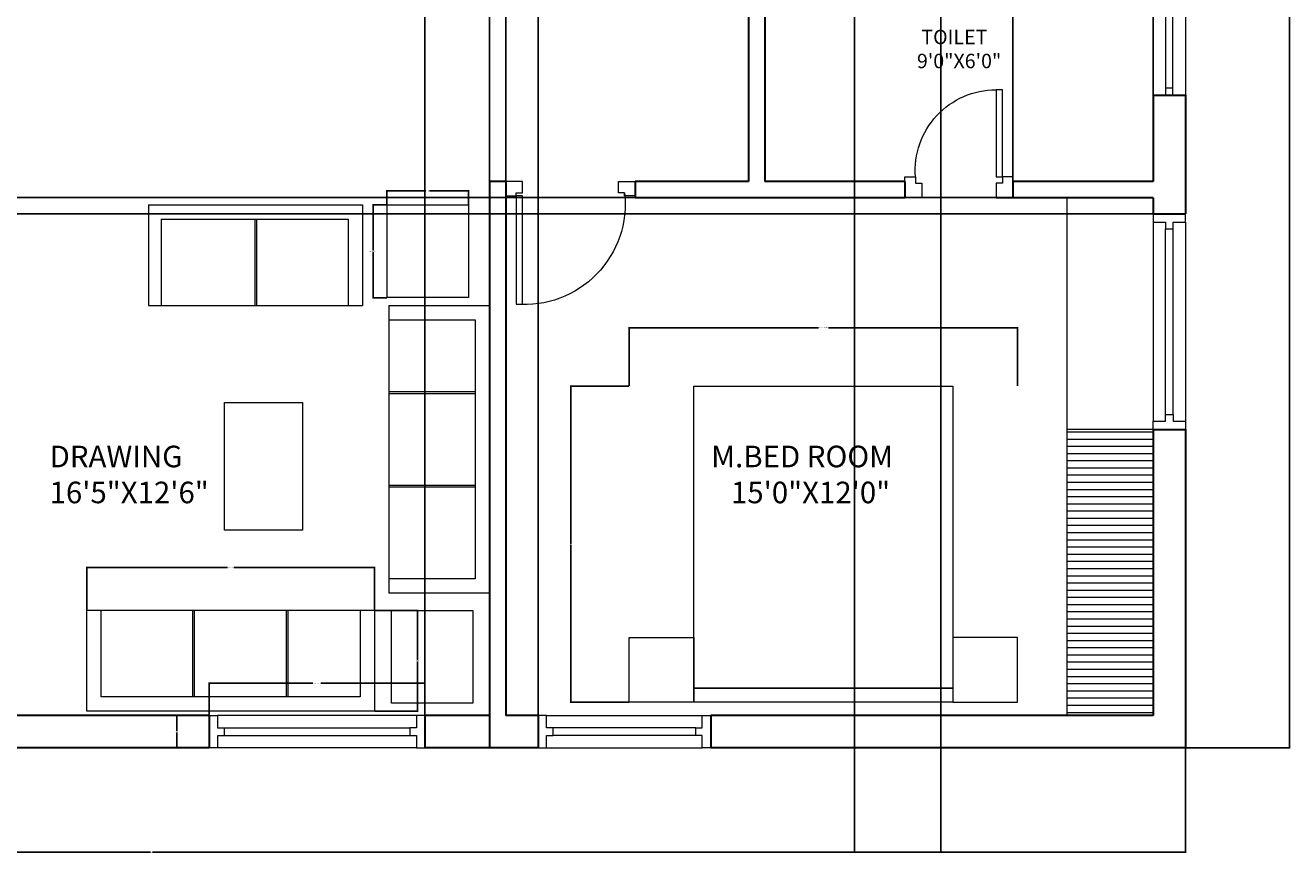
# Model space of a CAD drawing. Units: inches. Extents: x 2134 to 2768, y 715 to 1206.
# Tile 3 of 4: x 2416 to 2768, y 715 to 945. Entities that reach past the tile are written whole.
import ezdxf

# ---------------------------------------------------------------- set-up
doc = ezdxf.new("R2010")
doc.units = ezdxf.units.IN
for name, color, linetype, lineweight in [('A-ANNO-DIMS', 2, 'Continuous', 18), ('A-AREA-IDEN', 7, 'Continuous', 18), ('A-DOOR', 251, 'Continuous', 13), ('A-FLOR-CASE', 251, 'Continuous', 13), ('A-FLOR-CASE-PATT', 252, 'Continuous', 9), ('A-FURN', 251, 'Continuous', 13), ('A-WALL', 7, 'Continuous', 30), ('A-WINDOW', 251, 'Continuous', 13)]:
    doc.layers.add(name, color=color, linetype=linetype, lineweight=lineweight)
doc.styles.get("Standard").update_dxf_attribs({"font": 'arial.ttf'})
doc.dimstyles.get("Standard").update_dxf_attribs({"dimtxt": 0.18, "dimasz": 0.18, "dimexe": 0.18, "dimexo": 0.0625, "dimgap": 0.09, "dimtad": 0, "dimtih": 1, "dimtoh": 1, "dimdec": 4, "dimzin": 0, "dimdsep": 46, "dimtxsty": 'Standard', "dimcen": 0.09, "dimadec": 0, "dimazin": 0, "dimtfac": 1, "dimtdec": 4, "dimtofl": 0, "dimtmove": 0, "dimatfit": 3, "dimfxl": 1, "dimtolj": 1, "dimtzin": 0, "dimarcsym": 0})

# ---------------------------------------------------------------- blocks, each defined once
blk = doc.blocks.new('2 feet 6 inch door')
at = {"layer": 'A-DOOR'}
for points in [[(2.92, 5.83), (2.92, 30), (4.67, 30), (4.67, 5.83)], [(2.92, 4.08), (4.67, 4.08), (4.67, 0), (0, 0), (0, 5.83), (2.92, 5.83)], [(27.08, 5.83), (27.08, 4.08), (25.33, 4.08), (25.33, 0), (30, 0), (30, 5.83)]]:
    blk.add_lwpolyline(points, close=True, dxfattribs=at)
at = {"layer": 'A-DOOR', "ltscale": 0.1}
blk.add_arc((4.67, 7.52), 22.48, 355.6972, 90, dxfattribs=at)
blk = doc.blocks.new('ARCHITRAVE')
at = {"layer": 'A-DOOR'}
for p, q in [((0, 0), (0, 4)), ((0, 3.99), (2.92, 3.99)), ((2.92, 3.99), (2.92, 3.17)), ((4.67, 0), (0, 0)), ((2.92, 3.17), (4.67, 3.17)), ((4.67, 3.17), (4.67, 0))]:
    blk.add_line(p, q, dxfattribs=at)
blk = doc.blocks.new('3 FEET DOOR')
at = {"layer": 'A-DOOR'}
blk.add_lwpolyline([(-34.02, 3.98), (-34.02, 34.15), (-32.27, 34.15), (-32.27, 3.98)], close=True, dxfattribs=at)
at = {"layer": 'A-DOOR', "ltscale": 0.1}
blk.add_arc((-31.74, 6.19), 28.05, 353.8214, 94.662, dxfattribs=at)
at = {"layer": 'A-DOOR'}
blk.add_blockref('ARCHITRAVE', (-36.91, 0), dxfattribs=at)
at = {"layer": 'A-DOOR', "xscale": -1}
blk.add_blockref('ARCHITRAVE', (-0.93, 0), dxfattribs=at)
blk = doc.blocks.new('bed')
at = {"layer": 'A-FURN'}
for points in [[(3369.68, 925.24), (3297.68, 925.24), (3297.68, 1009.24), (3369.68, 1009.24)], [(3297.68, 921.32), (3279.68, 921.32), (3279.68, 939.32), (3297.68, 939.32)], [(3369.68, 921.32), (3387.68, 921.32), (3387.68, 939.32), (3369.68, 939.32)], [(3297.68, 925.24), (3369.68, 925.24), (3369.68, 921.32), (3297.68, 921.32)]]:
    blk.add_lwpolyline(points, close=True, dxfattribs=at)
blk = doc.blocks.new('WINDOW FRAME')
at = {"layer": 'A-WINDOW'}
for points in [[(4180.39, 4970.76), (4180.39, 4972.59), (4178.2, 4972.59), (4178.2, 4970.76)], [(4178.2, 4970.76), (4174.8, 4970.76), (4174.8, 4968.41), (4183.8, 4968.41), (4183.8, 4970.76), (4180.39, 4970.76)]]:
    blk.add_lwpolyline(points, dxfattribs=at)
blk = doc.blocks.new("4' window")
at = {"layer": 'A-WINDOW'}
for p, q in [((2.35, 9), (45.65, 9)), ((43.82, 5.59), (4.18, 5.59)), ((2.35, 0), (45.65, 0)), ((43.82, 3.41), (4.18, 3.41))]:
    blk.add_line(p, q, dxfattribs=at)
at = {"layer": 'A-WINDOW', "rotation": 270}
blk.add_blockref('WINDOW FRAME', (-4968.41, 4183.8), dxfattribs=at)
at = {"layer": 'A-WINDOW', "xscale": -1, "rotation": 90}
blk.add_blockref('WINDOW FRAME', (5016.41, 4183.8), dxfattribs=at)
blk = doc.blocks.new("5' door")
at = {"layer": 'A-WINDOW'}
for p, q in [((2.35, 9), (57.65, 9)), ((55.82, 5.59), (4.18, 5.59)), ((2.35, 0), (57.65, 0)), ((55.82, 3.41), (4.18, 3.41))]:
    blk.add_line(p, q, dxfattribs=at)
for points in [[(2.35, 5.59), (2.35, 9), (0, 9), (0, 0), (2.35, 0), (2.35, 3.41)], [(2.35, 3.41), (4.18, 3.41), (4.18, 5.59), (2.35, 5.59)]]:
    blk.add_lwpolyline(points, dxfattribs=at)
at = {"layer": 'A-WINDOW', "xscale": -1, "rotation": 90}
blk.add_blockref('WINDOW FRAME', (5028.41, 4183.8), dxfattribs=at)
blk = doc.blocks.new("2' ventilators")
at = {"layer": 'A-WINDOW'}
for p, q in [((24, 5.5), (0, 5.5)), ((1.93, 5.5), (1.93, 3.5)), ((22.07, 5.5), (22.07, 3.5))]:
    blk.add_line(p, q, dxfattribs=at)
for points in [[(0, 9), (24, 9), (24, 0), (0, 0), (0, 9)], [(24, 3.5), (0, 3.5)]]:
    blk.add_lwpolyline(points, dxfattribs=at)
blk = doc.blocks.new('SOFA-3-SEAT')
for p, q in [((0, 80), (0, 0)), ((0, 80), (28, 80)), ((28, 80), (28, 0)), ((0, 76), (24, 76)), ((24, 76), (24, 4)), ((24, 56), (0, 56)), ((24, 55.5), (0, 55.5)), ((24, 30), (0, 30)), ((24, 29.5), (0, 29.5)), ((24, 4), (0, 4)), ((28, 0), (0, 0))]:
    blk.add_line(p, q)
blk = doc.blocks.new('TABLE-END')
blk.add_lwpolyline([(0, 25.79), (22.63, 25.79), (22.63, 0), (0, 0)], close=True)
blk = doc.blocks.new('*D55')
at = {"layer": 'A-ANNO-DIMS', "color": 0, "lineweight": -2, "transparency": 16777216}
for p, q in [((2584.11, 844.79), (2584.11, 861.11)), ((2584.29, 860.93), (2636.72, 860.93)), ((2691.93, 860.93), (2639.49, 860.93)), ((2692.11, 844.79), (2692.11, 861.11))]:
    blk.add_line(p, q, dxfattribs=at)
at = {"layer": 'A-ANNO-DIMS', "color": 0, "transparency": 16777216}
for points in [[(2584.29, 860.96), (2584.29, 860.9), (2584.11, 860.93)], [(2691.93, 860.96), (2691.93, 860.9), (2692.11, 860.93)]]:
    blk.add_solid(points, dxfattribs=at)
at = {"layer": 'Defpoints', "color": 0, "transparency": 16777216}
for p in [(2692.11, 860.93), (2584.11, 844.73), (2692.11, 844.73)]:
    blk.add_point(p, dxfattribs=at)
at = {"layer": 'A-ANNO-DIMS', "color": 0, "transparency": 16777216, "insert": (2638.11, 860.93), "char_height": 0.18, "attachment_point": 5}
blk.add_mtext('\\A1;BED GROUP 108 TYP.', dxfattribs=at)
blk = doc.blocks.new('*D56')
at = {"layer": 'A-ANNO-DIMS', "color": 0, "lineweight": -2, "transparency": 16777216}
for p, q in [((2584.05, 844.73), (2567.73, 844.73)), ((2567.91, 844.55), (2567.91, 800.95)), ((2567.91, 756.98), (2567.91, 800.58)), ((2584.05, 756.8), (2567.73, 756.8))]:
    blk.add_line(p, q, dxfattribs=at)
at = {"layer": 'A-ANNO-DIMS', "color": 0, "transparency": 16777216}
for points in [[(2567.88, 844.55), (2567.94, 844.55), (2567.91, 844.73)], [(2567.88, 756.98), (2567.94, 756.98), (2567.91, 756.8)]]:
    blk.add_solid(points, dxfattribs=at)
at = {"layer": 'Defpoints', "color": 0, "transparency": 16777216}
for p in [(2567.91, 844.73), (2584.11, 844.73), (2584.11, 756.8)]:
    blk.add_point(p, dxfattribs=at)
at = {"layer": 'A-ANNO-DIMS', "color": 0, "transparency": 16777216, "insert": (2567.91, 800.77), "char_height": 0.18, "attachment_point": 5}
blk.add_mtext('\\A1;88 TYP.', dxfattribs=at)
blk = doc.blocks.new('*D61')
at = {"layer": 'A-ANNO-DIMS', "color": 0, "lineweight": -2, "transparency": 16777216}
for p, q in [((2467.29, 753.17), (2467.29, 762.29)), ((2467.47, 762.11), (2496.17, 762.11)), ((2527.11, 762.11), (2498.4, 762.11)), ((2527.29, 753.17), (2527.29, 762.29))]:
    blk.add_line(p, q, dxfattribs=at)
at = {"layer": 'A-ANNO-DIMS', "color": 0, "transparency": 16777216}
for points in [[(2467.47, 762.14), (2467.47, 762.08), (2467.29, 762.11)], [(2527.11, 762.14), (2527.11, 762.08), (2527.29, 762.11)]]:
    blk.add_solid(points, dxfattribs=at)
at = {"layer": 'Defpoints', "color": 0, "transparency": 16777216}
for p in [(2467.29, 762.11), (2467.29, 753.11), (2527.29, 753.11)]:
    blk.add_point(p, dxfattribs=at)
at = {"layer": 'A-ANNO-DIMS', "color": 0, "transparency": 16777216, "insert": (2497.29, 762.11), "char_height": 0.18, "attachment_point": 5}
blk.add_mtext('\\A1;GLAZING 60 TYP.', dxfattribs=at)
blk = doc.blocks.new('*D62')
at = {"layer": 'A-ANNO-DIMS', "color": 0, "lineweight": -2, "transparency": 16777216}
for p, q in [((2467.22, 753.11), (2458.11, 753.11)), ((2458.29, 752.93), (2458.29, 748.79)), ((2458.29, 744.29), (2458.29, 748.43)), ((2467.22, 744.11), (2458.11, 744.11))]:
    blk.add_line(p, q, dxfattribs=at)
at = {"layer": 'A-ANNO-DIMS', "color": 0, "transparency": 16777216}
for points in [[(2458.26, 752.93), (2458.32, 752.93), (2458.29, 753.11)], [(2458.26, 744.29), (2458.32, 744.29), (2458.29, 744.11)]]:
    blk.add_solid(points, dxfattribs=at)
at = {"layer": 'Defpoints', "color": 0, "transparency": 16777216}
for p in [(2467.29, 753.11), (2458.29, 744.11), (2467.29, 744.11)]:
    blk.add_point(p, dxfattribs=at)
at = {"layer": 'A-ANNO-DIMS', "color": 0, "transparency": 16777216, "insert": (2458.29, 748.61), "char_height": 0.18, "attachment_point": 5}
blk.add_mtext('\\A1;9 TYP.', dxfattribs=at)
blk = doc.blocks.new('*D65')
at = {"layer": 'A-ANNO-DIMS', "color": 0, "lineweight": -2, "transparency": 16777216}
for p, q in [((2433.29, 782.36), (2433.29, 794.47)), ((2433.47, 794.29), (2472.38, 794.29)), ((2513.11, 794.29), (2474.19, 794.29)), ((2513.29, 782.36), (2513.29, 794.47))]:
    blk.add_line(p, q, dxfattribs=at)
at = {"layer": 'A-ANNO-DIMS', "color": 0, "transparency": 16777216}
for points in [[(2433.47, 794.32), (2433.47, 794.26), (2433.29, 794.29)], [(2513.11, 794.32), (2513.11, 794.26), (2513.29, 794.29)]]:
    blk.add_solid(points, dxfattribs=at)
at = {"layer": 'Defpoints', "color": 0, "transparency": 16777216}
for p in [(2513.29, 794.29), (2433.29, 782.29), (2513.29, 782.29)]:
    blk.add_point(p, dxfattribs=at)
at = {"layer": 'A-ANNO-DIMS', "color": 0, "transparency": 16777216, "insert": (2473.29, 794.29), "char_height": 0.18, "attachment_point": 5}
blk.add_mtext('\\A1;SOFA 80 TYP.', dxfattribs=at)
blk = doc.blocks.new('*D66')
at = {"layer": 'A-ANNO-DIMS', "color": 0, "lineweight": -2, "transparency": 16777216}
for p, q in [((2513.35, 782.29), (2525.47, 782.29)), ((2525.29, 782.11), (2525.29, 768.48)), ((2525.29, 754.47), (2525.29, 768.11)), ((2513.35, 754.29), (2525.47, 754.29))]:
    blk.add_line(p, q, dxfattribs=at)
at = {"layer": 'A-ANNO-DIMS', "color": 0, "transparency": 16777216}
for points in [[(2525.26, 782.11), (2525.32, 782.11), (2525.29, 782.29)], [(2525.26, 754.47), (2525.32, 754.47), (2525.29, 754.29)]]:
    blk.add_solid(points, dxfattribs=at)
at = {"layer": 'Defpoints', "color": 0, "transparency": 16777216}
for p in [(2513.29, 782.29), (2513.29, 754.29), (2525.29, 754.29)]:
    blk.add_point(p, dxfattribs=at)
at = {"layer": 'A-ANNO-DIMS', "color": 0, "transparency": 16777216, "insert": (2525.29, 768.29), "char_height": 0.18, "attachment_point": 5}
blk.add_mtext('\\A1;28 TYP.', dxfattribs=at)
blk = doc.blocks.new('*D67')
at = {"layer": 'A-ANNO-DIMS', "color": 0, "lineweight": -2, "transparency": 16777216}
for p, q in [((2516.71, 895.1), (2512.72, 895.1)), ((2512.9, 894.92), (2512.9, 882.38)), ((2512.9, 869.48), (2512.9, 882.02)), ((2516.71, 869.3), (2512.72, 869.3))]:
    blk.add_line(p, q, dxfattribs=at)
at = {"layer": 'A-ANNO-DIMS', "color": 0, "transparency": 16777216}
for points in [[(2512.87, 894.92), (2512.93, 894.92), (2512.9, 895.1)], [(2512.87, 869.48), (2512.93, 869.48), (2512.9, 869.3)]]:
    blk.add_solid(points, dxfattribs=at)
at = {"layer": 'Defpoints', "color": 0, "transparency": 16777216}
for p in [(2512.9, 895.1), (2516.77, 895.1), (2516.77, 869.3)]:
    blk.add_point(p, dxfattribs=at)
at = {"layer": 'A-ANNO-DIMS', "color": 0, "transparency": 16777216, "insert": (2512.9, 882.2), "char_height": 0.18, "attachment_point": 5}
blk.add_mtext('\\A1;END TABLE 26 TYP.', dxfattribs=at)
blk = doc.blocks.new('*D68')
at = {"layer": 'A-ANNO-DIMS', "color": 0, "lineweight": -2, "transparency": 16777216}
for p, q in [((2516.77, 895.16), (2516.77, 899.15)), ((2516.95, 898.97), (2527.56, 898.97)), ((2539.22, 898.97), (2528.61, 898.97)), ((2539.4, 895.16), (2539.4, 899.15))]:
    blk.add_line(p, q, dxfattribs=at)
at = {"layer": 'A-ANNO-DIMS', "color": 0, "transparency": 16777216}
for points in [[(2516.95, 899), (2516.95, 898.94), (2516.77, 898.97)], [(2539.22, 899), (2539.22, 898.94), (2539.4, 898.97)]]:
    blk.add_solid(points, dxfattribs=at)
at = {"layer": 'Defpoints', "color": 0, "transparency": 16777216}
for p in [(2539.4, 898.97), (2516.77, 895.1), (2539.4, 895.1)]:
    blk.add_point(p, dxfattribs=at)
at = {"layer": 'A-ANNO-DIMS', "color": 0, "transparency": 16777216, "insert": (2528.09, 898.97), "char_height": 0.18, "attachment_point": 5}
blk.add_mtext('\\A1;23 TYP.', dxfattribs=at)
blk = doc.blocks.new('*D84')
at = {"layer": 'A-ANNO-DIMS', "color": 0, "lineweight": -2, "transparency": 16777216}
for p, q in [((2527.29, 753.17), (2527.29, 1205.74)), ((2527.47, 1205.56), (2536.08, 1205.56)), ((2545.11, 1205.56), (2536.5, 1205.56)), ((2545.29, 753.17), (2545.29, 1205.74))]:
    blk.add_line(p, q, dxfattribs=at)
at = {"layer": 'A-ANNO-DIMS', "color": 0, "transparency": 16777216}
for points in [[(2527.47, 1205.59), (2527.47, 1205.53), (2527.29, 1205.56)], [(2545.11, 1205.59), (2545.11, 1205.53), (2545.29, 1205.56)]]:
    blk.add_solid(points, dxfattribs=at)
at = {"layer": 'Defpoints', "color": 0, "transparency": 16777216}
for p in [(2545.29, 1205.56), (2527.29, 753.11), (2545.29, 753.11)]:
    blk.add_point(p, dxfattribs=at)
at = {"layer": 'A-ANNO-DIMS', "color": 0, "transparency": 16777216, "insert": (2536.29, 1205.56), "char_height": 0.18, "attachment_point": 5}
blk.add_mtext('\\A1;18', dxfattribs=at)
blk = doc.blocks.new('*D85')
at = {"layer": 'A-ANNO-DIMS', "color": 0, "lineweight": -2, "transparency": 16777216}
for p, q in [((2549.79, 753.17), (2549.79, 1205.74)), ((2549.97, 1205.56), (2554.14, 1205.56)), ((2558.61, 1205.56), (2554.44, 1205.56)), ((2558.79, 753.17), (2558.79, 1205.74))]:
    blk.add_line(p, q, dxfattribs=at)
at = {"layer": 'A-ANNO-DIMS', "color": 0, "transparency": 16777216}
for points in [[(2549.97, 1205.59), (2549.97, 1205.53), (2549.79, 1205.56)], [(2558.61, 1205.59), (2558.61, 1205.53), (2558.79, 1205.56)]]:
    blk.add_solid(points, dxfattribs=at)
at = {"layer": 'Defpoints', "color": 0, "transparency": 16777216}
for p in [(2558.79, 1205.56), (2549.79, 753.11), (2558.79, 753.11)]:
    blk.add_point(p, dxfattribs=at)
at = {"layer": 'A-ANNO-DIMS', "color": 0, "transparency": 16777216, "insert": (2554.29, 1205.56), "char_height": 0.18, "attachment_point": 5}
blk.add_mtext('\\A1;9', dxfattribs=at)
blk = doc.blocks.new('*D90')
at = {"layer": 'A-ANNO-DIMS', "color": 0, "lineweight": -2, "transparency": 16777216}
for p, q in [((2729.72, 897.11), (2134.66, 897.11)), ((2134.84, 896.93), (2134.84, 895.04)), ((2134.84, 892.79), (2134.84, 894.68)), ((2729.72, 892.61), (2134.66, 892.61))]:
    blk.add_line(p, q, dxfattribs=at)
at = {"layer": 'A-ANNO-DIMS', "color": 0, "transparency": 16777216}
for points in [[(2134.81, 896.93), (2134.87, 896.93), (2134.84, 897.11)], [(2134.81, 892.79), (2134.87, 892.79), (2134.84, 892.61)]]:
    blk.add_solid(points, dxfattribs=at)
at = {"layer": 'Defpoints', "color": 0, "transparency": 16777216}
for p in [(2729.79, 897.11), (2134.84, 892.61), (2729.79, 892.61)]:
    blk.add_point(p, dxfattribs=at)
at = {"layer": 'A-ANNO-DIMS', "color": 0, "transparency": 16777216, "insert": (2134.84, 894.86), "char_height": 0.18, "attachment_point": 5}
blk.add_mtext('\\A1;4.5', dxfattribs=at)
blk = doc.blocks.new('*D98')
at = {"layer": 'A-ANNO-DIMS', "color": 0, "lineweight": -2, "transparency": 16777216}
for p, q in [((2646.79, 1041.03), (2646.79, 714.98)), ((2670.79, 1041.03), (2670.79, 714.98)), ((2646.97, 715.16), (2658.57, 715.16)), ((2670.61, 715.16), (2659.01, 715.16))]:
    blk.add_line(p, q, dxfattribs=at)
at = {"layer": 'A-ANNO-DIMS', "color": 0, "transparency": 16777216}
for points in [[(2646.97, 715.19), (2646.97, 715.13), (2646.79, 715.16)], [(2670.61, 715.19), (2670.61, 715.13), (2670.79, 715.16)]]:
    blk.add_solid(points, dxfattribs=at)
at = {"layer": 'Defpoints', "color": 0, "transparency": 16777216}
for p in [(2646.79, 1041.09), (2670.79, 1041.09), (2670.79, 715.16)]:
    blk.add_point(p, dxfattribs=at)
at = {"layer": 'A-ANNO-DIMS', "color": 0, "transparency": 16777216, "insert": (2658.79, 715.16), "char_height": 0.18, "attachment_point": 5}
blk.add_mtext('\\A1;24', dxfattribs=at)
blk = doc.blocks.new('*D104')
at = {"layer": 'A-ANNO-DIMS', "color": 0, "lineweight": -2, "transparency": 16777216}
for p, q in [((2690.79, 901.67), (2690.79, 1205.74)), ((2690.97, 1205.56), (2710.07, 1205.56)), ((2729.61, 1205.56), (2710.51, 1205.56)), ((2729.79, 901.67), (2729.79, 1205.74))]:
    blk.add_line(p, q, dxfattribs=at)
at = {"layer": 'A-ANNO-DIMS', "color": 0, "transparency": 16777216}
for points in [[(2690.97, 1205.59), (2690.97, 1205.53), (2690.79, 1205.56)], [(2729.61, 1205.59), (2729.61, 1205.53), (2729.79, 1205.56)]]:
    blk.add_solid(points, dxfattribs=at)
at = {"layer": 'Defpoints', "color": 0, "transparency": 16777216}
for p in [(2729.79, 1205.56), (2690.79, 901.61), (2729.79, 901.61)]:
    blk.add_point(p, dxfattribs=at)
at = {"layer": 'A-ANNO-DIMS', "color": 0, "transparency": 16777216, "insert": (2710.29, 1205.56), "char_height": 0.18, "attachment_point": 5}
blk.add_mtext('\\A1;39', dxfattribs=at)
blk = doc.blocks.new('*D105')
at = {"layer": 'A-ANNO-DIMS', "color": 0, "lineweight": -2, "transparency": 16777216}
for p, q in [((2163.79, 897.04), (2163.79, 714.98)), ((2738.79, 744.04), (2738.79, 714.98)), ((2163.97, 715.16), (2451, 715.16)), ((2738.61, 715.16), (2451.58, 715.16))]:
    blk.add_line(p, q, dxfattribs=at)
at = {"layer": 'A-ANNO-DIMS', "color": 0, "transparency": 16777216}
for points in [[(2163.97, 715.19), (2163.97, 715.13), (2163.79, 715.16)], [(2738.61, 715.19), (2738.61, 715.13), (2738.79, 715.16)]]:
    blk.add_solid(points, dxfattribs=at)
at = {"layer": 'Defpoints', "color": 0, "transparency": 16777216}
for p in [(2163.79, 897.11), (2738.79, 744.11), (2738.79, 715.16)]:
    blk.add_point(p, dxfattribs=at)
at = {"layer": 'A-ANNO-DIMS', "color": 0, "transparency": 16777216, "insert": (2451.29, 715.16), "char_height": 0.18, "attachment_point": 5}
blk.add_mtext('\\A1;575', dxfattribs=at)
blk = doc.blocks.new('*D106')
at = {"layer": 'A-ANNO-DIMS', "color": 0, "lineweight": -2, "transparency": 16777216}
for p, q in [((2549.85, 1176.61), (2767.92, 1176.61)), ((2767.74, 1176.43), (2767.74, 960.54)), ((2767.74, 744.29), (2767.74, 960.18)), ((2738.85, 744.11), (2767.92, 744.11))]:
    blk.add_line(p, q, dxfattribs=at)
at = {"layer": 'A-ANNO-DIMS', "color": 0, "transparency": 16777216}
for points in [[(2767.71, 1176.43), (2767.77, 1176.43), (2767.74, 1176.61)], [(2767.71, 744.29), (2767.77, 744.29), (2767.74, 744.11)]]:
    blk.add_solid(points, dxfattribs=at)
at = {"layer": 'Defpoints', "color": 0, "transparency": 16777216}
for p in [(2549.79, 1176.61), (2767.74, 1176.61), (2738.79, 744.11)]:
    blk.add_point(p, dxfattribs=at)
at = {"layer": 'A-ANNO-DIMS', "color": 0, "transparency": 16777216, "insert": (2767.74, 960.36), "char_height": 0.18, "attachment_point": 5}
blk.add_mtext('\\A1;432.5', dxfattribs=at)

msp = doc.modelspace()

# ---------------------------------------------------------------- hatches: boundary and pattern name
at = {"layer": 'A-FLOR-CASE-PATT'}
h = msp.add_hatch(dxfattribs=at)
h.set_pattern_fill('_USER', color=256, scale=2, pattern_type=0)
h.set_pattern_definition([(0, (0, 0), (0, 2), [])])
h.paths.add_polyline_path([(2729.787, 832.607), (2705.787, 832.607), (2705.787, 753.107), (2729.787, 753.107)])

# ---------------------------------------------------------------- linework, layer by layer
at = {"layer": 'A-FLOR-CASE'}
for p, q in [((2705.787, 897.107), (2705.787, 753.107)), ((2729.787, 832.607), (2705.787, 832.607))]:
    msp.add_line(p, q, dxfattribs=at)
at = {"layer": 'A-FURN'}
for p, q in [((2450.494, 895.107), (2509.994, 895.107)), ((2450.494, 895.107), (2450.494, 867.107)), ((2509.994, 895.107), (2509.994, 867.107)), ((2453.994, 891.107), (2505.994, 891.107)), ((2453.994, 891.107), (2453.994, 867.107)), ((2479.994, 891.107), (2479.994, 867.107)), ((2480.494, 891.107), (2480.494, 867.107)), ((2505.994, 891.107), (2505.994, 867.107)), ((2450.494, 867.107), (2509.994, 867.107))]:
    msp.add_line(p, q, dxfattribs=at)
msp.add_lwpolyline([(2471.622, 840.153), (2493.275, 840.153), (2493.275, 804.677), (2471.622, 804.677)], close=True, dxfattribs=at)
at = {"layer": 'A-WALL'}
for p, q in [((2617.287, 973.607), (2617.287, 901.607)), ((2621.787, 973.607), (2621.787, 901.607)), ((2729.787, 925.607), (2738.787, 925.607)), ((2729.787, 925.607), (2729.787, 901.607)), ((2738.787, 925.607), (2738.787, 892.607)), ((2545.287, 901.607), (2545.287, 753.107)), ((2549.787, 901.607), (2545.287, 901.607)), ((2549.787, 901.607), (2549.787, 753.107)), ((2585.787, 901.607), (2585.787, 897.107)), ((2617.287, 901.607), (2585.787, 901.607)), ((2660.787, 901.607), (2621.787, 901.607)), ((2660.787, 901.607), (2660.787, 897.107)), ((2729.787, 901.607), (2690.787, 901.607)), ((2690.787, 901.607), (2690.787, 897.107)), ((2660.787, 897.107), (2585.787, 897.107)), ((2729.787, 897.107), (2690.787, 897.107)), ((2729.787, 897.107), (2729.787, 892.607)), ((2729.787, 892.607), (2738.787, 892.607)), ((2729.787, 832.607), (2738.787, 832.607)), ((2729.787, 832.607), (2729.787, 753.107)), ((2738.787, 832.607), (2738.787, 744.107)), ((2467.287, 753.107), (2408.287, 753.107)), ((2467.287, 753.107), (2467.287, 744.107)), ((2545.287, 753.107), (2527.287, 753.107)), ((2527.287, 753.107), (2527.287, 744.107)), ((2545.287, 753.107), (2545.287, 744.107)), ((2558.787, 753.107), (2549.787, 753.107)), ((2558.787, 753.107), (2558.787, 744.107)), ((2729.787, 753.107), (2606.787, 753.107)), ((2606.787, 753.107), (2606.787, 744.107)), ((2467.287, 744.107), (2408.287, 744.107)), ((2558.787, 744.107), (2527.287, 744.107)), ((2738.787, 744.107), (2606.787, 744.107))]:
    msp.add_line(p, q, dxfattribs=at)

# ---------------------------------------------------------------- block references
at = {"layer": 'A-DOOR', "xscale": -1}
msp.add_blockref('2 feet 6 inch door', (2690.787, 897.107), dxfattribs=at)
at = {"layer": 'A-DOOR', "xscale": -1, "rotation": 180}
msp.add_blockref('3 FEET DOOR', (2586.695, 901.607), dxfattribs=at)
at = {"layer": 'A-FURN'}
for name, p in [('TABLE-END', (2516.772, 869.305)), ('SOFA-3-SEAT', (2517.287, 787.107)), ('bed', (-695.575, -164.514)), ('TABLE-END', (2518.047, 756.519))]:
    msp.add_blockref(name, p, dxfattribs=at)
at = {"layer": 'A-FURN', "rotation": 270.0000000000003}
msp.add_blockref('SOFA-3-SEAT', (2433.287, 782.294), dxfattribs=at)
at = {"layer": 'A-WINDOW'}
for name, p, rotation in [("2' ventilators", (2729.787, 949.607), 270), ("5' door", (2729.787, 892.607), 270), ("5' door", (2527.287, 753.107), 180)]:
    msp.add_blockref(name, p, dxfattribs=dict(at, rotation=rotation))
msp.add_blockref("4' window", (2558.787, 744.107), dxfattribs=at)

# ---------------------------------------------------------------- texts
at = {"layer": 'A-AREA-IDEN', "attachment_point": 1}
for s, width, insert, char_height in [('  TOILET\\P 9\'0"X6\'0"', 55.72169, (2662.899, 943.781), 4), ('   DRAWING \\P   16\'5"X12\'6"', 143.74098, (2417.45, 828.141), 6), (' M.BED ROOM   \\P    15\'0"X12\'0"', 143.74098, (2605.079, 828.141), 6)]:
    msp.add_mtext_dynamic_manual_height_columns(s, width=width, gutter_width=12.5, heights=[0], dxfattribs=dict(at, insert=insert, char_height=char_height))

# ---------------------------------------------------------------- dimensions: what is measured, and where the dimension line sits
at = {"layer": 'A-ANNO-DIMS'}
for base, p1, p2, picture, middle in [((2545.287, 1205.557), (2527.287, 753.107), (2545.287, 753.107), '*D84', (2536.287, 1205.557)), ((2558.787, 1205.557), (2549.787, 753.107), (2558.787, 753.107), '*D85', (2554.287, 1205.557)), ((2729.787, 1205.557), (2690.787, 901.607), (2729.787, 901.607), '*D104', (2710.287, 1205.557)), ((2670.787, 715.157), (2646.787, 1041.091), (2670.787, 1041.091), '*D98', (2658.787, 715.157)), ((2738.787, 715.157), (2163.787, 897.107), (2738.787, 744.107), '*D105', (2451.287, 715.157))]:
    dim = msp.add_linear_dim(base=base, p1=p1, p2=p2, dimstyle='Standard', override={"dimdec": 0, "dimlfac": 1, "dimrnd": 0, "dimzin": 0, "dimdsep": 46, "dimlunit": 2}, dxfattribs=at)
    dim.commit()
    dim.dimension.update_dxf_attribs({"geometry": picture, "text_midpoint": middle})
for base, p1, p2, picture, middle in [((2767.737, 1176.607), (2738.787, 744.107), (2549.787, 1176.607), '*D106', (2767.737, 960.357)), ((2134.837, 892.607), (2729.787, 897.107), (2729.787, 892.607), '*D90', (2134.837, 894.857))]:
    dim = msp.add_linear_dim(base=base, p1=p1, p2=p2, angle=90, dimstyle='Standard', override={"dimdec": 1, "dimlfac": 1, "dimrnd": 0, "dimzin": 0, "dimdsep": 46, "dimlunit": 2}, dxfattribs=at)
    dim.commit()
    dim.dimension.update_dxf_attribs({"geometry": picture, "text_midpoint": middle})
for base, p1, p2, text, picture, middle in [((2539.398, 898.969), (2516.772, 895.1), (2539.398, 895.1), '<> TYP.', '*D68', (2528.085, 898.969)), ((2692.108, 860.931), (2584.108, 844.731), (2692.108, 844.731), 'BED GROUP <> TYP.', '*D55', (2638.108, 860.931))]:
    dim = msp.add_linear_dim(base=base, p1=p1, p2=p2, text=text, dimstyle='Standard', override={"dimdec": 0, "dimlfac": 1, "dimrnd": 0, "dimzin": 0, "dimdsep": 46, "dimlunit": 2}, dxfattribs=at)
    dim.commit()
    dim.dimension.update_dxf_attribs({"geometry": picture, "text_midpoint": middle})
for base, p1, p2, angle, text, picture, middle in [((2512.903, 895.1), (2516.772, 869.305), (2516.772, 895.1), 90, 'END TABLE <> TYP.', '*D67', (2512.903, 882.202)), ((2567.908, 844.731), (2584.108, 756.802), (2584.108, 844.731), 90, '<> TYP.', '*D56', (2567.908, 800.767)), ((2513.287, 794.294), (2433.287, 782.294), (2513.287, 782.294), 0, 'SOFA <> TYP.', '*D65', (2473.287, 794.294)), ((2525.287, 754.294), (2513.287, 782.294), (2513.287, 754.294), 270, '<> TYP.', '*D66', (2525.287, 768.294)), ((2467.287, 762.107), (2527.287, 753.107), (2467.287, 753.107), 180, 'GLAZING <> TYP.', '*D61', (2497.287, 762.107)), ((2458.287, 744.107), (2467.287, 753.107), (2467.287, 744.107), 270, '<> TYP.', '*D62', (2458.287, 748.607))]:
    dim = msp.add_linear_dim(base=base, p1=p1, p2=p2, angle=angle, text=text, dimstyle='Standard', override={"dimdec": 0, "dimlfac": 1, "dimrnd": 0, "dimzin": 0, "dimdsep": 46, "dimlunit": 2}, dxfattribs=at)
    dim.commit()
    dim.dimension.update_dxf_attribs({"geometry": picture, "text_midpoint": middle})

doc.saveas('drawing.dxf')
